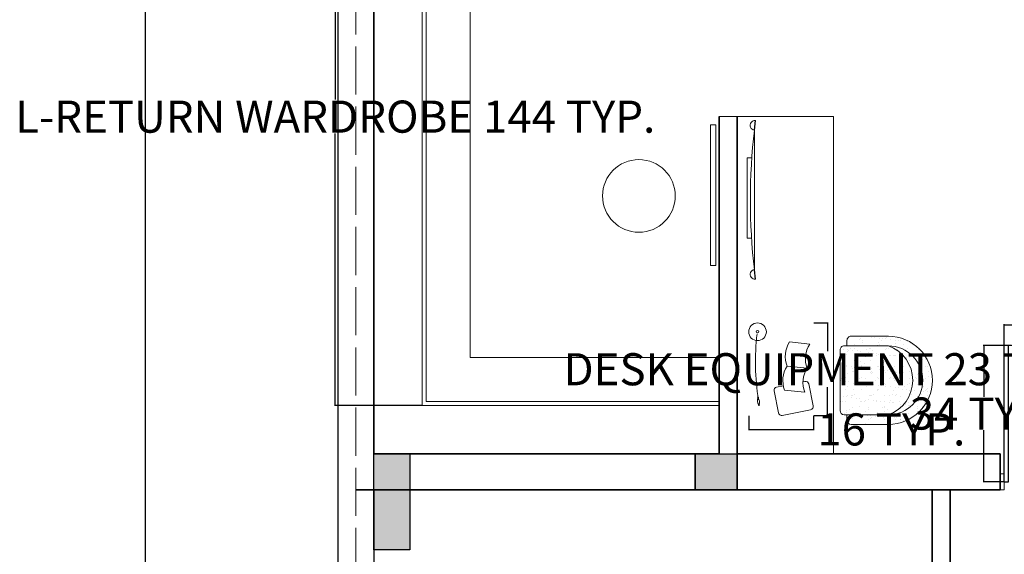
# Model space of a CAD drawing. Units: inches. Extents: x -48 to 50072, y 0 to 21068.
# Tile 66 of 75: x 680 to 925, y 915 to 1049. Entities that reach past the tile are written whole.
import ezdxf

# ---------------------------------------------------------------- set-up
doc = ezdxf.new("R2010")
doc.units = ezdxf.units.IN
doc.header["$MEASUREMENT"] = 0
doc.linetypes.add('ACAD_ISO02W100', pattern=[15, 12, -3])
for name, color, linetype, lineweight in [('A-ANNO-DIMS', 2, 'Continuous', 18), ('A-COLS', 1, 'Continuous', 35), ('A-DOOR', 4, 'Continuous', 18), ('A-EQPM', 8, 'Continuous', 18), ('A-FLOR-CASE', 9, 'Continuous', 18), ('A-WALL', 7, 'Continuous', 35), ('C-PROP', 7, 'Continuous', 25), ('C-PROP-REF', 32, 'ACAD_ISO02W100', 13), ('FURNITURE', 44, 'Continuous', 18)]:
    doc.layers.add(name, color=color, linetype=linetype, lineweight=lineweight)
doc.styles.get("Standard").update_dxf_attribs({"font": 'arial.ttf'})
doc.dimstyles.get("Standard").update_dxf_attribs({"dimtxt": 8, "dimasz": 0.18, "dimexe": 0.18, "dimexo": 0.0625, "dimgap": 0.09, "dimtad": 0, "dimtih": 1, "dimtoh": 1, "dimdec": 1, "dimzin": 0, "dimdsep": 46, "dimlunit": 4, "dimtxsty": 'Standard', "dimblk": 'ARCHTICK', "dimcen": 0.09, "dimadec": 0, "dimazin": 0, "dimtfac": 1, "dimtdec": 1, "dimtofl": 0, "dimtmove": 0, "dimatfit": 3, "dimldrblk": 'ARCHTICK', "dimfxl": 1, "dimtolj": 1, "dimtzin": 0, "dimarcsym": 0})

# ---------------------------------------------------------------- blocks, each defined once
blk = doc.blocks.new('BKUHJKKUG')
at = {"layer": 'Defpoints'}
for p, q in [((179.52, 862.77), (179.52, 896.77)), ((180.52, 862.77), (180.52, 896.76)), ((179.52, 862.77), (180.52, 862.77))]:
    blk.add_line(p, q, dxfattribs=at)
blk.add_arc((179.52, 862.77), 34, 0, 90, dxfattribs=at)
at = {"insert": (190.84, 874.8), "char_height": 2.9183, "attachment_point": 1}
blk.add_mtext_dynamic_manual_height_columns('\\pxqc;WOODEN ^JDOOR', width=9.6242, gutter_width=14.59, heights=[0], dxfattribs=at)
blk = doc.blocks.new('bnniku')
at = {"layer": 'Defpoints'}
h = blk.add_hatch(color=256, dxfattribs=at)
h.dxf.hatch_style = 1
h.paths.add_polyline_path([(767.55, 1114.04), (758.55, 1114.04), (758.55, 1090.04), (767.55, 1090.04)])
for p, q in [((758.55, 1114.04), (767.55, 1114.04)), ((758.55, 1090.04), (758.55, 1114.04)), ((767.55, 1114.04), (767.55, 1090.04)), ((767.55, 1090.04), (758.55, 1090.04))]:
    blk.add_line(p, q, dxfattribs=at)
blk = doc.blocks.new('khll')
at = {"layer": 'Defpoints'}
h = blk.add_hatch(color=256, dxfattribs=at)
h.dxf.hatch_style = 1
h.paths.add_polyline_path([(105.52, 1025.77), (116.02, 1025.77), (116.02, 1034.77), (105.52, 1034.77)])
for p, q in [((105.52, 1025.77), (105.52, 1034.77)), ((116.02, 1025.77), (116.02, 1034.77))]:
    blk.add_line(p, q)
for p, q in [((105.52, 1034.77), (116.02, 1034.77)), ((105.52, 1025.77), (116.02, 1025.77))]:
    blk.add_line(p, q, dxfattribs=at)
blk = doc.blocks.new('CHAIR-STUDY')
for p, q in [((1.73, 20.94), (1.73, 19.57)), ((1.74, 20.38, 13.84), (1.74, 20.38, 13.84)), ((2.76, 21.97), (12.03, 21.96)), ((3.55, 19.84, 13.84), (3.55, 19.84, 13.84)), ((3.67, 21.9, 13.84), (3.67, 21.9, 13.84)), ((4.87, 21.05, 13.84), (4.87, 21.05, 13.84)), ((5.15, 21.3, 13.84), (5.15, 21.3, 13.84)), ((5.52, 20.9, 13.84), (5.52, 20.9, 13.84)), ((5.63, 20.39, 13.84), (5.63, 20.39, 13.84)), ((6.44, 21.95, 13.84), (6.44, 21.95, 13.84)), ((7.77, 21.75, 13.84), (7.77, 21.75, 13.84)), ((8.5, 21.68, 13.84), (8.5, 21.68, 13.84)), ((9.44, 19.71, 13.84), (9.44, 19.71, 13.84)), ((9.61, 20.34, 13.84), (9.61, 20.34, 13.84)), ((9.72, 19.97, 13.84), (9.72, 19.97, 13.84)), ((9.74, 21.52, 13.84), (9.74, 21.52, 13.84)), ((10.25, 20.89, 13.84), (10.25, 20.89, 13.84)), ((10.53, 21.41, 13.84), (10.53, 21.41, 13.84)), ((11.24, 21.36, 13.84), (11.24, 21.36, 13.84)), ((11.66, 21.77, 13.84), (11.66, 21.77, 13.84)), ((12.59, 21.14, 13.84), (12.59, 21.14, 13.84)), ((13.71, 20.2, 13.84), (13.71, 20.2, 13.84)), ((13.83, 20.98, 13.84), (13.83, 20.98, 13.84)), ((14.62, 20.87, 13.84), (14.62, 20.87, 13.84)), ((14.99, 20.88, 13.84), (14.99, 20.88, 13.84)), ((15.81, 20.02, 13.84), (15.81, 20.02, 13.84)), ((16.68, 20.6, 13.84), (16.68, 20.6, 13.84)), ((17.6, 20.21, 13.84), (17.6, 20.21, 13.84)), ((0.01, 18.54), (0, 3.44)), ((0.15, 18.84, 13.84), (0.15, 18.84, 13.84)), ((0.94, 18.74, 13.84), (0.94, 18.74, 13.84)), ((1.04, 19.57), (12.03, 19.56)), ((1.64, 17.45, 13.84), (1.64, 17.45, 13.84)), ((1.76, 18.19, 13.84), (1.76, 18.19, 13.84)), ((1.87, 18.57, 13.84), (1.87, 18.57, 13.84)), ((2.04, 18.45, 13.84), (2.04, 18.45, 13.84)), ((2.51, 18.98, 13.84), (2.51, 18.98, 13.84)), ((3.01, 18.47, 13.84), (3.01, 18.47, 13.84)), ((3.57, 18.97, 13.84), (3.57, 18.97, 13.84)), ((4.24, 18.3, 13.84), (4.24, 18.3, 13.84)), ((5.03, 18.2, 13.84), (5.03, 18.2, 13.84)), ((5.53, 17.47, 13.84), (5.53, 17.47, 13.84)), ((6.6, 18.56, 13.84), (6.6, 18.56, 13.84)), ((7.1, 17.93, 13.84), (7.1, 17.93, 13.84)), ((7.24, 18.97, 13.84), (7.24, 18.97, 13.84)), ((7.68, 18.82, 13.84), (7.68, 18.82, 13.84)), ((8.12, 18.5, 13.84), (8.12, 18.5, 13.84)), ((8.34, 17.77, 13.84), (8.34, 17.77, 13.84)), ((9.13, 17.66, 13.84), (9.13, 17.66, 13.84)), ((9.51, 17.42, 13.84), (9.51, 17.42, 13.84)), ((11.19, 17.39, 13.84), (11.19, 17.39, 13.84)), ((11.33, 18.56, 13.84), (11.33, 18.56, 13.84)), ((11.57, 18.84, 13.84), (11.57, 18.84, 13.84)), ((11.97, 18.96, 13.84), (11.97, 18.96, 13.84)), ((12.43, 17.23, 13.84), (12.43, 17.23, 13.84)), ((12.69, 17.17, 13.84), (12.69, 17.17, 13.84)), ((13.62, 17.27, 13.84), (13.62, 17.27, 13.84)), ((14.01, 18.38, 13.84), (14.01, 18.38, 13.84)), ((14.29, 18.64, 13.84), (14.29, 18.64, 13.84)), ((15.54, 18.79, 13.84), (15.54, 18.79, 13.84)), ((16.07, 18.55, 13.84), (16.07, 18.55, 13.84)), ((16.71, 18.96, 13.84), (16.71, 18.96, 13.84)), ((17.5, 17.29, 13.84), (17.5, 17.29, 13.84)), ((18.86, 17.3, 13.84), (18.86, 17.3, 13.84)), ((19.65, 18.64, 13.84), (19.65, 18.64, 13.84)), ((0.44, 16.98, 13.84), (0.44, 16.98, 13.84)), ((0.64, 14.77, 13.84), (0.64, 14.77, 13.84)), ((1.28, 15.17, 13.84), (1.28, 15.17, 13.84)), ((1.61, 14.72, 13.84), (1.61, 14.72, 13.84)), ((3.48, 16.04, 13.84), (3.48, 16.04, 13.84)), ((4.29, 17.09, 13.84), (4.29, 17.09, 13.84)), ((5.01, 15.65, 13.84), (5.01, 15.65, 13.84)), ((5.37, 14.76, 13.84), (5.37, 14.76, 13.84)), ((6.01, 15.17, 13.84), (6.01, 15.17, 13.84)), ((6.33, 16.86, 13.84), (6.33, 16.86, 13.84)), ((6.61, 17.12, 13.84), (6.61, 17.12, 13.84)), ((7.58, 15.89, 13.84), (7.58, 15.89, 13.84)), ((9.02, 17.09, 13.84), (9.02, 17.09, 13.84)), ((10.1, 14.75, 13.84), (10.1, 14.75, 13.84)), ((10.75, 15.16, 13.84), (10.75, 15.16, 13.84)), ((10.9, 15.52, 13.84), (10.9, 15.52, 13.84)), ((11.18, 15.78, 13.84), (11.18, 15.78, 13.84)), ((11.47, 15.91, 13.84), (11.47, 15.91, 13.84)), ((13.22, 17.12, 13.84), (13.22, 17.12, 13.84)), ((13.76, 17.08, 13.84), (13.76, 17.08, 13.84)), ((14.84, 14.74, 13.84), (14.84, 14.74, 13.84)), ((15.28, 16.85, 13.84), (15.28, 16.85, 13.84)), ((15.45, 15.86, 13.84), (15.45, 15.86, 13.84)), ((15.48, 15.15, 13.84), (15.48, 15.15, 13.84)), ((16.52, 16.69, 13.84), (16.52, 16.69, 13.84)), ((17.26, 15.83, 13.84), (17.26, 15.83, 13.84)), ((17.31, 16.58, 13.84), (17.31, 16.58, 13.84)), ((18.49, 17.07, 13.84), (18.49, 17.07, 13.84)), ((18.58, 17.05, 13.84), (18.58, 17.05, 13.84)), ((19.37, 16.31, 13.84), (19.37, 16.31, 13.84)), ((19.55, 15.71, 13.84), (19.55, 15.71, 13.84)), ((19.57, 14.73, 13.84), (19.57, 14.73, 13.84)), ((20.21, 15.14, 13.84), (20.21, 15.14, 13.84)), ((20.61, 16.15, 13.84), (20.61, 16.15, 13.84)), ((21.4, 16.05, 13.84), (21.4, 16.05, 13.84)), ((1.55, 14.52, 13.84), (1.55, 14.52, 13.84)), ((1.89, 12.79, 13.84), (1.89, 12.79, 13.84)), ((2.84, 14.55, 13.84), (2.84, 14.55, 13.84)), ((3.06, 13.29, 13.84), (3.06, 13.29, 13.84)), ((3.21, 14, 13.84), (3.21, 14, 13.84)), ((3.38, 13.11, 13.84), (3.38, 13.11, 13.84)), ((3.49, 14.26, 13.84), (3.49, 14.26, 13.84)), ((3.63, 14.45, 13.84), (3.63, 14.45, 13.84)), ((5.44, 14.54, 13.84), (5.44, 14.54, 13.84)), ((5.7, 14.18, 13.84), (5.7, 14.18, 13.84)), ((6.93, 14.01, 13.84), (6.93, 14.01, 13.84)), ((7.49, 12.96, 13.84), (7.49, 12.96, 13.84)), ((7.72, 13.91, 13.84), (7.72, 13.91, 13.84)), ((7.78, 12.67, 13.84), (7.78, 12.67, 13.84)), ((7.8, 13.28, 13.84), (7.8, 13.28, 13.84)), ((8.06, 12.93, 13.84), (8.06, 12.93, 13.84)), ((9.41, 14.49, 13.84), (9.41, 14.49, 13.84)), ((9.58, 14.31, 13.84), (9.58, 14.31, 13.84)), ((9.79, 13.64, 13.84), (9.79, 13.64, 13.84)), ((11.03, 13.48, 13.84), (11.03, 13.48, 13.84)), ((11.37, 12.98, 13.84), (11.37, 12.98, 13.84)), ((11.82, 13.37, 13.84), (11.82, 13.37, 13.84)), ((12.53, 13.27, 13.84), (12.53, 13.27, 13.84)), ((13.52, 14.34, 13.84), (13.52, 14.34, 13.84)), ((13.88, 13.1, 13.84), (13.88, 13.1, 13.84)), ((14.14, 12.98, 13.84), (14.14, 12.98, 13.84)), ((15.12, 12.94, 13.84), (15.12, 12.94, 13.84)), ((15.35, 12.93, 13.84), (15.35, 12.93, 13.84)), ((15.47, 14.19, 13.84), (15.47, 14.19, 13.84)), ((15.75, 14.45, 13.84), (15.75, 14.45, 13.84)), ((15.91, 12.83, 13.84), (15.91, 12.83, 13.84)), ((17.26, 13.26, 13.84), (17.26, 13.26, 13.84)), ((17.41, 14.36, 13.84), (17.41, 14.36, 13.84)), ((17.97, 12.56, 13.84), (17.97, 12.56, 13.84)), ((19.21, 12.4, 13.84), (19.21, 12.4, 13.84)), ((19.46, 12.78, 13.84), (19.46, 12.78, 13.84)), ((20, 12.29, 13.84), (20, 12.29, 13.84)), ((20.04, 12.86, 13.84), (20.04, 12.86, 13.84)), ((20.32, 13.11, 13.84), (20.32, 13.11, 13.84)), ((21.39, 14.31, 13.84), (21.39, 14.31, 13.84)), ((21.83, 14.5, 13.84), (21.83, 14.5, 13.84)), ((22, 13.25, 13.84), (22, 13.25, 13.84)), ((0.05, 11.37, 13.84), (0.05, 11.37, 13.84)), ((0.1, 11.15, 13.84), (0.1, 11.15, 13.84)), ((0.21, 10.96, 13.84), (0.21, 10.96, 13.84)), ((0.38, 11.41, 13.84), (0.38, 11.41, 13.84)), ((1.44, 10.8, 13.84), (1.44, 10.8, 13.84)), ((1.45, 11.59, 13.84), (1.45, 11.59, 13.84)), ((2.23, 10.7, 13.84), (2.23, 10.7, 13.84)), ((3.28, 10.18, 13.84), (3.28, 10.18, 13.84)), ((4.14, 10.95, 13.84), (4.14, 10.95, 13.84)), ((4.3, 10.43, 13.84), (4.3, 10.43, 13.84)), ((4.67, 9.81, 13.84), (4.67, 9.81, 13.84)), ((4.78, 11.36, 13.84), (4.78, 11.36, 13.84)), ((4.95, 10.07, 13.84), (4.95, 10.07, 13.84)), ((5.34, 11.61, 13.84), (5.34, 11.61, 13.84)), ((5.53, 10.26, 13.84), (5.53, 10.26, 13.84)), ((6.32, 10.16, 13.84), (6.32, 10.16, 13.84)), ((6.46, 11.46, 13.84), (6.46, 11.46, 13.84)), ((7.39, 10.04, 13.84), (7.39, 10.04, 13.84)), ((8.39, 9.89, 13.84), (8.39, 9.89, 13.84)), ((8.88, 10.94, 13.84), (8.88, 10.94, 13.84)), ((9.32, 11.56, 13.84), (9.32, 11.56, 13.84)), ((9.52, 11.35, 13.84), (9.52, 11.35, 13.84)), ((11.03, 10.12, 13.84), (11.03, 10.12, 13.84)), ((11.28, 10.05, 13.84), (11.28, 10.05, 13.84)), ((12.35, 11.34, 13.84), (12.35, 11.34, 13.84)), ((12.63, 11.59, 13.84), (12.63, 11.59, 13.84)), ((13.42, 11.41, 13.84), (13.42, 11.41, 13.84)), ((13.61, 10.93, 13.84), (13.61, 10.93, 13.84)), ((14.25, 11.34, 13.84), (14.25, 11.34, 13.84)), ((15.26, 10, 13.84), (15.26, 10, 13.84)), ((16.92, 10, 13.84), (16.92, 10, 13.84)), ((17.2, 10.26, 13.84), (17.2, 10.26, 13.84)), ((17.31, 11.43, 13.84), (17.31, 11.43, 13.84)), ((18.34, 10.93, 13.84), (18.34, 10.93, 13.84)), ((18.71, 11.64, 13.84), (18.71, 11.64, 13.84)), ((18.99, 11.33, 13.84), (18.99, 11.33, 13.84)), ((19.36, 9.86, 13.84), (19.36, 9.86, 13.84)), ((21.29, 11.38, 13.84), (21.29, 11.38, 13.84)), ((22.06, 12.02, 13.84), (22.06, 12.02, 13.84)), ((1.36, 8.66, 13.84), (1.36, 8.66, 13.84)), ((1.84, 9.48, 13.84), (1.84, 9.48, 13.84)), ((3.34, 8.6, 13.84), (3.34, 8.6, 13.84)), ((3.56, 7.55, 13.84), (3.56, 7.55, 13.84)), ((5.24, 8.68, 13.84), (5.24, 8.68, 13.84)), ((6.57, 9.47, 13.84), (6.57, 9.47, 13.84)), ((8.29, 7.55, 13.84), (8.29, 7.55, 13.84)), ((9.22, 8.63, 13.84), (9.22, 8.63, 13.84)), ((9.24, 8.48, 13.84), (9.24, 8.48, 13.84)), ((9.52, 8.74, 13.84), (9.52, 8.74, 13.84)), ((9.62, 9.72, 13.84), (9.62, 9.72, 13.84)), ((10.41, 9.62, 13.84), (10.41, 9.62, 13.84)), ((11.3, 9.46, 13.84), (11.3, 9.46, 13.84)), ((12.48, 9.35, 13.84), (12.48, 9.35, 13.84)), ((13.02, 7.54, 13.84), (13.02, 7.54, 13.84)), ((13.33, 8.48, 13.84), (13.33, 8.48, 13.84)), ((13.72, 9.19, 13.84), (13.72, 9.19, 13.84)), ((14.09, 7.4, 13.84), (14.09, 7.4, 13.84)), ((14.51, 9.08, 13.84), (14.51, 9.08, 13.84)), ((15.6, 8.79, 13.84), (15.6, 8.79, 13.84)), ((16.04, 9.46, 13.84), (16.04, 9.46, 13.84)), ((16.57, 8.81, 13.84), (16.57, 8.81, 13.84)), ((17.22, 8.5, 13.84), (17.22, 8.5, 13.84)), ((17.76, 7.53, 13.84), (17.76, 7.53, 13.84)), ((17.81, 8.65, 13.84), (17.81, 8.65, 13.84)), ((18.6, 8.54, 13.84), (18.6, 8.54, 13.84)), ((20.17, 7.46, 13.84), (20.17, 7.46, 13.84)), ((20.66, 8.27, 13.84), (20.66, 8.27, 13.84)), ((20.77, 9.45, 13.84), (20.77, 9.45, 13.84)), ((21.2, 8.45, 13.84), (21.2, 8.45, 13.84)), ((21.49, 8.67, 13.84), (21.49, 8.67, 13.84)), ((21.77, 8.92, 13.84), (21.77, 8.92, 13.84)), ((21.9, 8.11, 13.84), (21.9, 8.11, 13.84)), ((0.04, 7.05, 13.84), (0.04, 7.05, 13.84)), ((0.23, 5.75, 13.84), (0.23, 5.75, 13.84)), ((0.61, 5.68, 13.84), (0.61, 5.68, 13.84)), ((0.83, 6.95, 13.84), (0.83, 6.95, 13.84)), ((1.26, 5.73, 13.84), (1.26, 5.73, 13.84)), ((1.55, 6.96, 13.84), (1.55, 6.96, 13.84)), ((1.83, 7.22, 13.84), (1.83, 7.22, 13.84)), ((2.9, 6.68, 13.84), (2.9, 6.68, 13.84)), ((2.92, 7.15, 13.84), (2.92, 7.15, 13.84)), ((3.19, 7.25, 13.84), (3.19, 7.25, 13.84)), ((4.13, 6.51, 13.84), (4.13, 6.51, 13.84)), ((4.92, 6.41, 13.84), (4.92, 6.41, 13.84)), ((5.15, 5.75, 13.84), (5.15, 5.75, 13.84)), ((5.34, 5.67, 13.84), (5.34, 5.67, 13.84)), ((6.12, 5.63, 13.84), (6.12, 5.63, 13.84)), ((6.4, 5.88, 13.84), (6.4, 5.88, 13.84)), ((6.99, 6.14, 13.84), (6.99, 6.14, 13.84)), ((7.29, 7.11, 13.84), (7.29, 7.11, 13.84)), ((7.65, 7.14, 13.84), (7.65, 7.14, 13.84)), ((7.91, 7.27, 13.84), (7.91, 7.27, 13.84)), ((8.22, 5.97, 13.84), (8.22, 5.97, 13.84)), ((9.01, 5.87, 13.84), (9.01, 5.87, 13.84)), ((9.13, 5.7, 13.84), (9.13, 5.7, 13.84)), ((10.08, 5.66, 13.84), (10.08, 5.66, 13.84)), ((11.08, 5.6, 13.84), (11.08, 5.6, 13.84)), ((11.18, 7.13, 13.84), (11.18, 7.13, 13.84)), ((12.31, 5.44, 13.84), (12.31, 5.44, 13.84)), ((12.38, 7.13, 13.84), (12.38, 7.13, 13.84)), ((12.48, 5.93, 13.84), (12.48, 5.93, 13.84)), ((13.1, 5.33, 13.84), (13.1, 5.33, 13.84)), ((13.23, 5.55, 13.84), (13.23, 5.55, 13.84)), ((13.81, 7.15, 13.84), (13.81, 7.15, 13.84)), ((14.81, 5.65, 13.84), (14.81, 5.65, 13.84)), ((15.16, 7.07, 13.84), (15.16, 7.07, 13.84)), ((15.17, 5.06, 13.84), (15.17, 5.06, 13.84)), ((17.12, 7.12, 13.84), (17.12, 7.12, 13.84)), ((17.12, 5.57, 13.84), (17.12, 5.57, 13.84)), ((18.37, 5.81, 13.84), (18.37, 5.81, 13.84)), ((18.65, 6.07, 13.84), (18.65, 6.07, 13.84)), ((19.27, 6.93, 13.84), (19.27, 6.93, 13.84)), ((19.54, 5.64, 13.84), (19.54, 5.64, 13.84)), ((21.1, 5.52, 13.84), (21.1, 5.52, 13.84)), ((21.85, 7.11, 13.84), (21.85, 7.11, 13.84)), ((1.16, 2.8, 13.84), (1.16, 2.8, 13.84)), ((1.49, 2.92, 13.84), (1.49, 2.92, 13.84)), ((1.69, 3.34, 13.84), (1.69, 3.34, 13.84)), ((2.33, 3.75, 13.84), (2.33, 3.75, 13.84)), ((2.73, 2.76, 13.84), (2.73, 2.76, 13.84)), ((3.01, 2.77, 13.84), (3.01, 2.77, 13.84)), ((3.09, 4.33, 13.84), (3.09, 4.33, 13.84)), ((3.29, 3.03, 13.84), (3.29, 3.03, 13.84)), ((3.52, 2.66, 13.84), (3.52, 2.66, 13.84)), ((4.8, 4.41, 13.84), (4.8, 4.41, 13.84)), ((5.05, 2.82, 13.84), (5.05, 2.82, 13.84)), ((6.42, 3.33, 13.84), (6.42, 3.33, 13.84)), ((7.06, 3.74, 13.84), (7.06, 3.74, 13.84)), ((7.2, 4.18, 13.84), (7.2, 4.18, 13.84)), ((9.03, 2.77, 13.84), (9.03, 2.77, 13.84)), ((9.37, 3.08, 13.84), (9.37, 3.08, 13.84)), ((10.69, 4.29, 13.84), (10.69, 4.29, 13.84)), ((10.97, 4.55, 13.84), (10.97, 4.55, 13.84)), ((11.09, 4.2, 13.84), (11.09, 4.2, 13.84)), ((11.16, 3.32, 13.84), (11.16, 3.32, 13.84)), ((11.8, 3.73, 13.84), (11.8, 3.73, 13.84)), ((13.14, 2.62, 13.84), (13.14, 2.62, 13.84)), ((15.07, 4.15, 13.84), (15.07, 4.15, 13.84)), ((15.26, 2.96, 13.84), (15.26, 2.96, 13.84)), ((15.54, 3.21, 13.84), (15.54, 3.21, 13.84)), ((15.89, 3.31, 13.84), (15.89, 3.31, 13.84)), ((16.41, 4.9, 13.84), (16.41, 4.9, 13.84)), ((16.53, 3.72, 13.84), (16.53, 3.72, 13.84)), ((17.02, 2.64, 13.84), (17.02, 2.64, 13.84)), ((17.05, 4.6, 13.84), (17.05, 4.6, 13.84)), ((17.2, 4.79, 13.84), (17.2, 4.79, 13.84)), ((19.17, 4, 13.84), (19.17, 4, 13.84)), ((19.26, 4.52, 13.84), (19.26, 4.52, 13.84)), ((20.5, 4.36, 13.84), (20.5, 4.36, 13.84)), ((1.03, 2.41), (12.01, 2.4)), ((1.72, 2.41), (1.71, 1.04)), ((2.74, 0.01), (12.01, 0)), ((3, 1.4, 13.84), (3, 1.4, 13.84)), ((4.11, 1.86, 13.84), (4.11, 1.86, 13.84)), ((5.59, 2.39, 13.84), (5.59, 2.39, 13.84)), ((6.25, 0.23, 13.84), (6.25, 0.23, 13.84)), ((6.82, 2.22, 13.84), (6.82, 2.22, 13.84)), ((7.1, 1.25, 13.84), (7.1, 1.25, 13.84)), ((7.57, 1.44, 13.84), (7.57, 1.44, 13.84)), ((7.61, 2.12, 13.84), (7.61, 2.12, 13.84)), ((7.85, 1.69, 13.84), (7.85, 1.69, 13.84)), ((8.85, 1.85, 13.84), (8.85, 1.85, 13.84)), ((9.68, 1.85, 13.84), (9.68, 1.85, 13.84)), ((10.91, 1.68, 13.84), (10.91, 1.68, 13.84)), ((10.99, 1.27, 13.84), (10.99, 1.27, 13.84)), ((11.7, 1.58, 13.84), (11.7, 1.58, 13.84)), ((12.14, 0.1, 13.84), (12.14, 0.1, 13.84)), ((12.42, 0.36, 13.84), (12.42, 0.36, 13.84)), ((13.58, 1.84, 13.84), (13.58, 1.84, 13.84)), ((13.77, 1.31, 13.84), (13.77, 1.31, 13.84)), ((13.94, 1.75, 13.84), (13.94, 1.75, 13.84)), ((14.97, 1.22, 13.84), (14.97, 1.22, 13.84)), ((15, 1.15, 13.84), (15, 1.15, 13.84)), ((15.8, 1.04, 13.84), (15.8, 1.04, 13.84))]:
    blk.add_line(p, q)
for centre, radius, start, end in [((2.76, 20.94), 1.03, 89.9486, 179.9486), ((12.02, 10.98), 10.98, 359.9486, 89.9486), ((1.04, 18.54), 1.03, 89.9486, 179.9486), ((9.02, 10.98), 9.09, 289.2386, 70.6585), ((12.02, 10.98), 8.58, 359.9486, 89.9486), ((12.02, 10.98), 10.98, 269.9486, 359.9486), ((12.02, 10.98), 8.58, 269.9486, 359.9486), ((1.03, 3.44), 1.03, 179.9486, 269.9486), ((2.74, 1.04), 1.03, 179.9486, 269.9486)]:
    blk.add_arc(centre, radius, start, end)
blk = doc.blocks.new('DESK-ACCESSORIES')
for p, q in [((10.18, 18.3), (15.19, 17.78)), ((9.56, 12.3), (14.56, 11.78)), ((6.96, 7.08), (8.64, 7.41)), ((13.5, 8.38), (14.02, 8.49)), ((14.96, 7.86), (16.06, 2.37)), ((7.43, 0.64), (6.33, 6.13)), ((13.94, 5.81), (8.93, 6.33)), ((15.43, 1.43), (8.37, 0.02))]:
    blk.add_line(p, q)
for centre, radius, start, end in [((2.2, 20.84), 2.2, 90, 270), ((2.2, 20.84), 2.2, 270, 90), ((63.85, 13.23), 62.16, 173.4513, 188.6305), ((2.2, 20.84), 0.3, 90, 270), ((2.2, 20.84), 0.3, 270, 90), ((15.87, 14.66), 6.76, 147.37, 200.7442), ((20.88, 14.14), 6.76, 147.37, 200.7442), ((15.03, 8.7), 6.54, 146.9045, 201.2097), ((20.04, 8.18), 6.54, 146.9045, 201.2097), ((14.18, 7.7), 0.8, 11.3025, 101.3025), ((7.12, 6.29), 0.8, 101.3025, 191.3025), ((4, 3.71), 1.82, 157.356, 216.9378), ((2.33, 4.39), 0.12, 90, 270), ((0.87, 3.31), 1.82, 337.356, 36.9378), ((2.33, 4.39), 0.12, 270, 90), ((2.54, 2.6), 0.12, 90, 270), ((2.54, 2.6), 0.12, 270, 90), ((8.21, 0.8), 0.8, 191.3025, 281.3025), ((15.27, 2.21), 0.8, 281.3025, 11.3025)]:
    blk.add_arc(centre, radius, start, end)
blk = doc.blocks.new('DISPLAY-FLAT-PANEL')
for p, q in [((1.73, 37.17), (2.01, 39.54)), ((1.83, 37.19), (2.11, 39.53)), ((1.83, 2.35), (1.83, 37.19)), ((1.83, 37.19), (1.83, 37.19)), ((1.2, 30.3), (0, 30.3)), ((0, 30.3), (0, 10.23)), ((0, 10.23), (1.13, 10.23)), ((1.73, 2.37), (2.01, 0)), ((1.83, 2.35), (2.11, 0.01))]:
    blk.add_line(p, q)
for centre, radius, start, end in [((1.97, 38.34), 1.2, 83.3215, 263.5313), ((153.03, 19.77), 152.2, 173.4285, 186.5715), ((1.97, 1.2), 1.2, 96.4687, 276.6785)]:
    blk.add_arc(centre, radius, start, end)
blk = doc.blocks.new('WARDROBE-L-RETURN')
for p, q in [((0, 144), (0, 0)), ((1, 144), (1, 1)), ((12, 144), (12, 12)), ((74, 12), (12, 12)), ((74, 1), (1, 1)), ((74, 0), (0, 0))]:
    blk.add_line(p, q)
blk = doc.blocks.new('_ArchTick')
at = {"color": 0, "linetype": 'ByBlock', "const_width": 0.15}
blk.add_lwpolyline([(-0.5, -0.5), (0.5, 0.5)], dxfattribs=at)
blk = doc.blocks.new('*D66')
at = {"layer": 'A-ANNO-DIMS', "color": 0, "lineweight": -2, "transparency": 16777216}
for p, q in [((924.76, 967.53), (924.76, 972.74)), ((924.76, 972.56), (958.76, 972.56)), ((958.76, 967.53), (958.76, 972.74)), ((958.76, 972.56), (958.94, 972.56))]:
    blk.add_line(p, q, dxfattribs=at)
at = {"layer": 'Defpoints', "color": 0, "transparency": 16777216}
for p in [(958.76, 972.56), (924.76, 967.46), (958.76, 967.46)]:
    blk.add_point(p, dxfattribs=at)
at = {"layer": 'A-ANNO-DIMS', "color": 0, "lineweight": -2, "transparency": 16777216, "xscale": 0.18, "yscale": 0.18, "zscale": 0.18, "rotation": 180}
blk.add_blockref('_ArchTick', (924.76, 972.56), dxfattribs=at)
at = {"layer": 'A-ANNO-DIMS', "color": 0, "lineweight": -2, "transparency": 16777216, "xscale": 0.18, "yscale": 0.18, "zscale": 0.18}
blk.add_blockref('_ArchTick', (958.76, 972.56), dxfattribs=at)
at = {"layer": 'A-ANNO-DIMS', "color": 0, "transparency": 16777216, "insert": (1027.07, 972.56), "char_height": 8, "attachment_point": 5}
blk.add_mtext('\\A1;BEDROOM DOOR 34 TYP.', dxfattribs=at)
blk = doc.blocks.new('*D67')
at = {"layer": 'A-ANNO-DIMS', "color": 0, "lineweight": -2, "transparency": 16777216}
for p, q in [((924.7, 967.46), (919.48, 967.46)), ((919.66, 967.46), (919.66, 954.64)), ((919.66, 933.46), (919.66, 946.29)), ((924.7, 933.46), (919.48, 933.46))]:
    blk.add_line(p, q, dxfattribs=at)
at = {"layer": 'Defpoints', "color": 0, "transparency": 16777216}
for p in [(919.66, 967.46), (924.76, 967.46), (924.76, 933.46)]:
    blk.add_point(p, dxfattribs=at)
at = {"layer": 'A-ANNO-DIMS', "color": 0, "lineweight": -2, "transparency": 16777216, "xscale": 0.18, "yscale": 0.18, "zscale": 0.18}
for p, rotation in [((919.66, 967.46), 90), ((919.66, 933.46), 270)]:
    blk.add_blockref('_ArchTick', p, dxfattribs=dict(at, rotation=rotation))
at = {"layer": 'A-ANNO-DIMS', "color": 0, "transparency": 16777216, "insert": (919.66, 950.46), "char_height": 8, "attachment_point": 5}
blk.add_mtext('\\A1;34 TYP.', dxfattribs=at)
blk = doc.blocks.new('*D82')
at = {"layer": 'A-ANNO-DIMS', "color": 0, "lineweight": -2, "transparency": 16777216}
for p, q in [((877.31, 973.04), (880.89, 973.04)), ((880.71, 973.04), (880.71, 965.98)), ((880.71, 949.97), (880.71, 957.04)), ((877.31, 949.97), (880.89, 949.97))]:
    blk.add_line(p, q, dxfattribs=at)
at = {"layer": 'Defpoints', "color": 0, "transparency": 16777216}
for p in [(877.25, 973.04), (880.71, 973.04), (877.25, 949.97)]:
    blk.add_point(p, dxfattribs=at)
at = {"layer": 'A-ANNO-DIMS', "color": 0, "lineweight": -2, "transparency": 16777216, "xscale": 0.18, "yscale": 0.18, "zscale": 0.18}
for p, rotation in [((880.71, 973.04), 90), ((880.71, 949.97), 270)]:
    blk.add_blockref('_ArchTick', p, dxfattribs=dict(at, rotation=rotation))
at = {"layer": 'A-ANNO-DIMS', "color": 0, "transparency": 16777216, "insert": (880.71, 961.51), "char_height": 8, "attachment_point": 5}
blk.add_mtext('\\A1;DESK EQUIPMENT 23 TYP.', dxfattribs=at)
blk = doc.blocks.new('*D83')
at = {"layer": 'A-ANNO-DIMS', "color": 0, "lineweight": -2, "transparency": 16777216}
for p, q in [((861.11, 949.91), (861.11, 946.33)), ((877.25, 949.91), (877.25, 946.33)), ((861.11, 946.51), (877.25, 946.51)), ((877.25, 946.51), (877.43, 946.51))]:
    blk.add_line(p, q, dxfattribs=at)
at = {"layer": 'Defpoints', "color": 0, "transparency": 16777216}
for p in [(861.11, 949.97), (877.25, 949.97), (877.25, 946.51)]:
    blk.add_point(p, dxfattribs=at)
at = {"layer": 'A-ANNO-DIMS', "color": 0, "lineweight": -2, "transparency": 16777216, "xscale": 0.18, "yscale": 0.18, "zscale": 0.18, "rotation": 180}
blk.add_blockref('_ArchTick', (861.11, 946.51), dxfattribs=at)
at = {"layer": 'A-ANNO-DIMS', "color": 0, "lineweight": -2, "transparency": 16777216, "xscale": 0.18, "yscale": 0.18, "zscale": 0.18}
blk.add_blockref('_ArchTick', (877.25, 946.51), dxfattribs=at)
at = {"layer": 'A-ANNO-DIMS', "color": 0, "transparency": 16777216, "insert": (896.62, 946.51), "char_height": 8, "attachment_point": 5}
blk.add_mtext('\\A1;16 TYP.', dxfattribs=at)
blk = doc.blocks.new('*D102')
at = {"layer": 'A-ANNO-DIMS', "color": 0, "lineweight": -2, "transparency": 16777216}
for p, q in [((779.7, 1096.46), (757.98, 1096.46)), ((758.16, 1096.46), (758.16, 1028.69)), ((758.16, 952.46), (758.16, 1020.23)), ((779.7, 952.46), (757.98, 952.46))]:
    blk.add_line(p, q, dxfattribs=at)
at = {"layer": 'Defpoints', "color": 0, "transparency": 16777216}
for p in [(758.16, 1096.46), (779.76, 1096.46), (779.76, 952.46)]:
    blk.add_point(p, dxfattribs=at)
at = {"layer": 'A-ANNO-DIMS', "color": 0, "lineweight": -2, "transparency": 16777216, "xscale": 0.18, "yscale": 0.18, "zscale": 0.18}
for p, rotation in [((758.16, 1096.46), 90), ((758.16, 952.46), 270)]:
    blk.add_blockref('_ArchTick', p, dxfattribs=dict(at, rotation=rotation))
at = {"layer": 'A-ANNO-DIMS', "color": 0, "transparency": 16777216, "insert": (758.16, 1024.46), "char_height": 8, "attachment_point": 5}
blk.add_mtext('\\A1;L-RETURN WARDROBE 144 TYP.', dxfattribs=at)
blk = doc.blocks.new('*D130')
at = {"layer": 'A-ANNO-DIMS', "color": 0, "lineweight": -2, "transparency": 16777216}
for p, q in [((758.7, 1241.46), (710.63, 1241.46)), ((710.81, 1241.46), (710.81, 767.29)), ((710.81, 284.76), (710.81, 758.94)), ((758.7, 284.76), (710.63, 284.76))]:
    blk.add_line(p, q, dxfattribs=at)
at = {"layer": 'Defpoints', "color": 0, "transparency": 16777216}
for p in [(710.81, 1241.46), (758.76, 1241.46), (758.76, 284.76)]:
    blk.add_point(p, dxfattribs=at)
at = {"layer": 'A-ANNO-DIMS', "color": 0, "lineweight": -2, "transparency": 16777216, "xscale": 0.18, "yscale": 0.18, "zscale": 0.18}
for p, rotation in [((710.81, 1241.46), 90), ((710.81, 284.76), 270)]:
    blk.add_blockref('_ArchTick', p, dxfattribs=dict(at, rotation=rotation))
at = {"layer": 'A-ANNO-DIMS', "color": 0, "transparency": 16777216, "insert": (710.81, 763.11), "char_height": 8, "attachment_point": 5}
blk.add_mtext('\\A1;956.7', dxfattribs=at)

msp = doc.modelspace()

# ---------------------------------------------------------------- linework, layer by layer
at = {"layer": 'A-DOOR'}
for p, q in [((923.761, 935.464), (924.761, 935.464)), ((924.761, 935.464), (924.761, 931.464)), ((923.761, 931.464), (924.761, 931.464))]:
    msp.add_line(p, q, dxfattribs=at)
at = {"layer": 'A-FLOR-CASE'}
for p, q in [((882.261, 1024.464), (853.761, 1024.464)), ((882.261, 940.464), (882.261, 1024.464))]:
    msp.add_line(p, q, dxfattribs=at)
at = {"layer": 'A-WALL'}
for p, q in [((767.761, 1096.464), (767.761, 940.464)), ((853.761, 940.464), (853.761, 1024.464)), ((858.261, 940.464), (858.261, 1024.464)), ((853.761, 940.464), (767.761, 940.464)), ((923.761, 940.464), (858.261, 940.464)), ((923.761, 940.464), (923.761, 931.464)), ((923.761, 931.464), (763.261, 931.464)), ((906.761, 931.464), (906.761, 757.464)), ((911.261, 931.464), (911.261, 748.464))]:
    msp.add_line(p, q, dxfattribs=at)
at = {"layer": 'C-PROP'}
for p, q in [((758.761, 1241.464), (758.761, 284.764)), ((767.761, 931.464), (767.761, 293.764))]:
    msp.add_line(p, q, dxfattribs=at)
at = {"layer": 'C-PROP-REF'}
msp.add_line((763.261, 1236.964), (763.261, 284.764), dxfattribs=at)
at = {"layer": 'FURNITURE'}
msp.add_lwpolyline([(851.625, 1022.404), (852.93, 1022.404), (852.93, 987.325), (851.625, 987.325)], close=True, dxfattribs=at)
msp.add_circle((833.771, 1004.704), 9.049, dxfattribs=at)

# ---------------------------------------------------------------- block references
at = {"layer": 'A-COLS'}
for name, p in [('bnniku', (9.209, -173.573)), ('khll', (742.244, -94.311))]:
    msp.add_blockref(name, p, dxfattribs=at)
at = {"layer": 'A-DOOR'}
msp.add_blockref('BKUHJKKUG', (745.244, 70.689), dxfattribs=at)
at = {"layer": 'A-EQPM'}
msp.add_blockref('DISPLAY-FLAT-PANEL', (860.706, 983.932), dxfattribs=at)
at = {"layer": 'A-FLOR-CASE'}
msp.add_blockref('WARDROBE-L-RETURN', (779.761, 952.464), dxfattribs=at)
at = {"layer": 'FURNITURE'}
for name, p in [('DESK-ACCESSORIES', (861.107, 950)), ('CHAIR-STUDY', (883.855, 947.765))]:
    msp.add_blockref(name, p, dxfattribs=at)

# ---------------------------------------------------------------- dimensions: what is measured, and where the dimension line sits
at = {"layer": 'A-ANNO-DIMS'}
dim = msp.add_linear_dim(base=(710.811, 1241.464), p1=(758.761, 284.764), p2=(758.761, 1241.464), angle=90, dimstyle='Standard', override={"dimdec": 1, "dimlfac": 1, "dimrnd": 0, "dimzin": 0, "dimdsep": 46, "dimlunit": 2}, dxfattribs=at)
dim.commit()
dim.dimension.update_dxf_attribs({"geometry": '*D130', "text_midpoint": (710.811, 763.114)})
for base, p1, p2, text, picture, middle in [((758.161, 1096.464), (779.761, 952.464), (779.761, 1096.464), 'L-RETURN WARDROBE <> TYP.', '*D102', (758.161, 1024.464)), ((880.711, 973.042), (877.251, 949.974), (877.251, 973.042), 'DESK EQUIPMENT <> TYP.', '*D82', (880.711, 961.508)), ((919.661, 967.464), (924.761, 933.464), (924.761, 967.464), '<> TYP.', '*D67', (919.661, 950.464))]:
    dim = msp.add_linear_dim(base=base, p1=p1, p2=p2, angle=90, text=text, dimstyle='Standard', override={"dimdec": 0, "dimlfac": 1, "dimrnd": 0, "dimzin": 0, "dimdsep": 46, "dimlunit": 2}, dxfattribs=at)
    dim.commit()
    dim.dimension.update_dxf_attribs({"geometry": picture, "text_midpoint": middle})
for base, p1, p2, text, picture, middle in [((958.761, 972.564), (924.761, 967.464), (958.761, 967.464), 'BEDROOM DOOR <> TYP.', '*D66', (1027.066, 972.564)), ((877.251, 946.514), (861.107, 949.974), (877.251, 949.974), '<> TYP.', '*D83', (896.615, 946.514))]:
    dim = msp.add_linear_dim(base=base, p1=p1, p2=p2, text=text, dimstyle='Standard', override={"dimdec": 0, "dimlfac": 1, "dimrnd": 0, "dimzin": 0, "dimdsep": 46, "dimlunit": 2}, dxfattribs=at)
    dim.commit()
    dim.dimension.update_dxf_attribs({"geometry": picture, "text_midpoint": middle})

doc.saveas('drawing.dxf')
